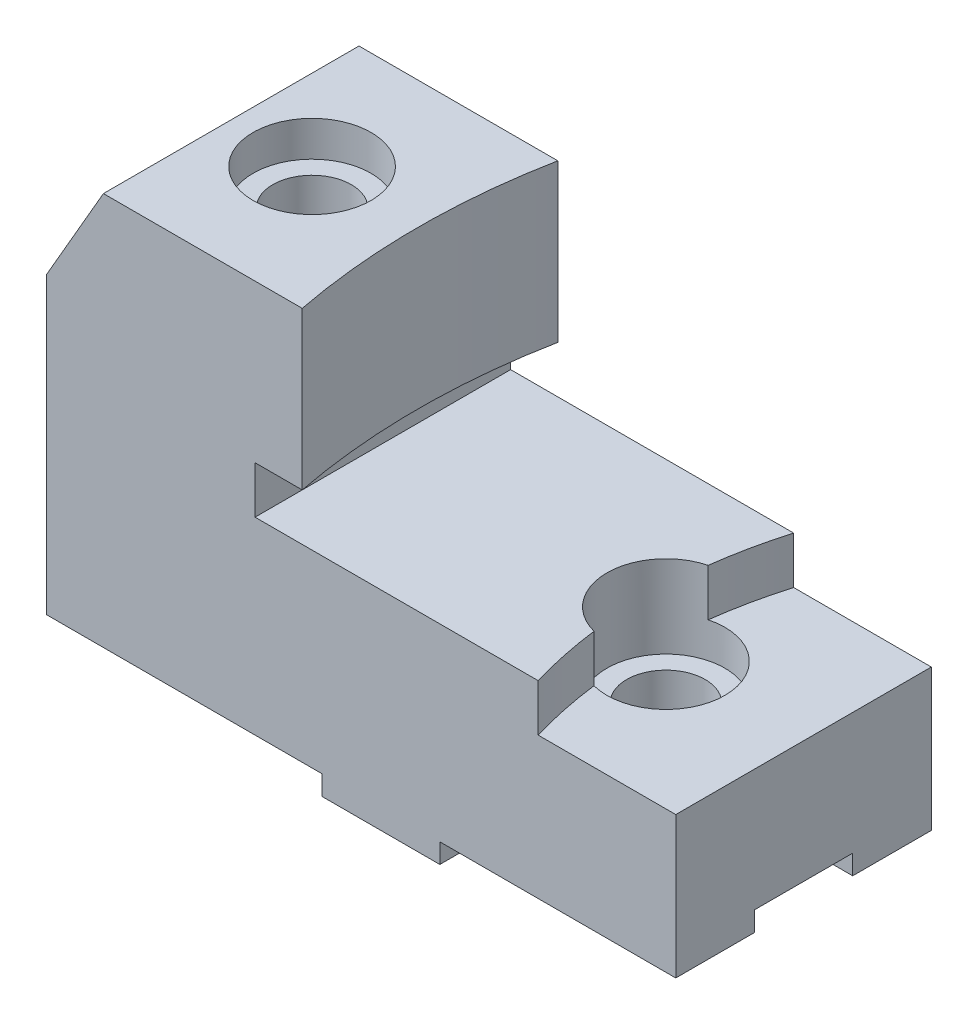
ISO-10303-21;
HEADER;
FILE_DESCRIPTION(('STEP AP214'),'2;1');
FILE_NAME('part.step','',(''),(''),'','','');
FILE_SCHEMA(('AUTOMOTIVE_DESIGN { 1 0 10303 214 1 1 1 1 }'));
ENDSEC;
DATA;
#1=APPLICATION_CONTEXT('core data for automotive mechanical design processes');
#2=APPLICATION_PROTOCOL_DEFINITION('international standard','automotive_design',2000,#1);
#3=PRODUCT_CONTEXT('',#1,'mechanical');
#4=PRODUCT('Part','Part','',(#3));
#5=PRODUCT_RELATED_PRODUCT_CATEGORY('part','',(#4));
#6=PRODUCT_DEFINITION_FORMATION('','',#4);
#7=PRODUCT_DEFINITION_CONTEXT('part definition',#1,'design');
#8=PRODUCT_DEFINITION('design','',#6,#7);
#9=PRODUCT_DEFINITION_SHAPE('','',#8);
#10=(LENGTH_UNIT() NAMED_UNIT(*) SI_UNIT(.MILLI.,.METRE.));
#11=(NAMED_UNIT(*) PLANE_ANGLE_UNIT() SI_UNIT($,.RADIAN.));
#12=(NAMED_UNIT(*) SI_UNIT($,.STERADIAN.) SOLID_ANGLE_UNIT());
#13=UNCERTAINTY_MEASURE_WITH_UNIT(LENGTH_MEASURE(1.E-05),#10,'distance_accuracy_value','');
#14=(GEOMETRIC_REPRESENTATION_CONTEXT(3) GLOBAL_UNCERTAINTY_ASSIGNED_CONTEXT((#13)) GLOBAL_UNIT_ASSIGNED_CONTEXT((#10,
#11,#12)) REPRESENTATION_CONTEXT('',''));
#15=CARTESIAN_POINT('',(0.,0.,0.));
#16=DIRECTION('',(0.,0.,1.));
#17=DIRECTION('',(1.,0.,0.));
#18=AXIS2_PLACEMENT_3D('',#15,#16,#17);
#19=CARTESIAN_POINT('',(235.312057364551,-289.269119345812,32.5));
#20=DIRECTION('',(0.,1.,0.));
#21=DIRECTION('',(-1.,0.,0.));
#22=AXIS2_PLACEMENT_3D('',#19,#20,#21);
#23=CYLINDRICAL_SURFACE('',#22,115.);
#24=CARTESIAN_POINT('',(235.312057364551,35.9999999999999,32.5));
#25=DIRECTION('',(0.,-1.,0.));
#26=DIRECTION('',(1.,0.,0.));
#27=AXIS2_PLACEMENT_3D('',#24,#25,#26);
#28=CIRCLE('',#27,115.);
#29=CARTESIAN_POINT('',(121.232279499362,36.,47.0191005998674));
#30=VERTEX_POINT('',#29);
#31=CARTESIAN_POINT('',(125.,36.,65.));
#32=VERTEX_POINT('',#31);
#33=EDGE_CURVE('E268',#30,#32,#28,.F.);
#34=ORIENTED_EDGE('',*,*,#33,.F.);
#35=DIRECTION('',(0.,1.,0.));
#36=VECTOR('',#35,1.);
#37=CARTESIAN_POINT('',(121.232279499362,42.,47.0191005998674));
#38=LINE('',#37,#36);
#39=CARTESIAN_POINT('',(121.232279499362,47.9999999999999,47.0191005998674));
#40=VERTEX_POINT('',#39);
#41=EDGE_CURVE('E479',#30,#40,#38,.T.);
#42=ORIENTED_EDGE('',*,*,#41,.T.);
#43=CARTESIAN_POINT('',(235.312057364551,47.9999999999998,32.5));
#44=DIRECTION('',(0.,1.,0.));
#45=DIRECTION('',(-1.,0.,0.));
#46=AXIS2_PLACEMENT_3D('',#43,#44,#45);
#47=CIRCLE('',#46,115.);
#48=CARTESIAN_POINT('',(125.,47.9999999999999,65.));
#49=VERTEX_POINT('',#48);
#50=EDGE_CURVE('E261',#40,#49,#47,.T.);
#51=ORIENTED_EDGE('',*,*,#50,.T.);
#52=DIRECTION('',(0.,1.,0.));
#53=VECTOR('',#52,1.);
#54=CARTESIAN_POINT('',(125.,48.,65.));
#55=LINE('',#54,#53);
#56=EDGE_CURVE('E332',#32,#49,#55,.T.);
#57=ORIENTED_EDGE('',*,*,#56,.F.);
#58=EDGE_LOOP('',(#34,#42,#51,#57));
#59=FACE_BOUND('',#58,.T.);
#60=ADVANCED_FACE('F39',(#59),#23,.F.);
#61=CARTESIAN_POINT('',(70.,0.,65.));
#62=DIRECTION('',(0.,1.,0.));
#63=DIRECTION('',(-1.,0.,0.));
#64=AXIS2_PLACEMENT_3D('',#61,#62,#63);
#65=PLANE('',#64);
#66=DIRECTION('',(0.,0.,-1.));
#67=VECTOR('',#66,1.);
#68=CARTESIAN_POINT('',(0.,0.,65.));
#69=LINE('',#68,#67);
#70=CARTESIAN_POINT('',(0.,0.,65.));
#71=VERTEX_POINT('',#70);
#72=CARTESIAN_POINT('',(0.,0.,45.));
#73=VERTEX_POINT('',#72);
#74=EDGE_CURVE('E217',#71,#73,#69,.T.);
#75=ORIENTED_EDGE('',*,*,#74,.T.);
#76=DIRECTION('',(1.,0.,0.));
#77=VECTOR('',#76,1.);
#78=CARTESIAN_POINT('',(70.,0.,45.));
#79=LINE('',#78,#77);
#80=CARTESIAN_POINT('',(70.,0.,45.));
#81=VERTEX_POINT('',#80);
#82=EDGE_CURVE('E179',#73,#81,#79,.T.);
#83=ORIENTED_EDGE('',*,*,#82,.T.);
#84=DIRECTION('',(0.,0.,-1.));
#85=VECTOR('',#84,1.);
#86=CARTESIAN_POINT('',(70.,0.,65.));
#87=LINE('',#86,#85);
#88=CARTESIAN_POINT('',(70.,0.,65.));
#89=VERTEX_POINT('',#88);
#90=EDGE_CURVE('E48',#89,#81,#87,.T.);
#91=ORIENTED_EDGE('',*,*,#90,.F.);
#92=DIRECTION('',(1.,0.,0.));
#93=VECTOR('',#92,1.);
#94=CARTESIAN_POINT('',(70.,0.,65.));
#95=LINE('',#94,#93);
#96=EDGE_CURVE('E213',#71,#89,#95,.T.);
#97=ORIENTED_EDGE('',*,*,#96,.F.);
#98=EDGE_LOOP('',(#75,#83,#91,#97));
#99=FACE_BOUND('',#98,.T.);
#100=ADVANCED_FACE('F368',(#99),#65,.F.);
#101=CARTESIAN_POINT('',(70.,0.,65.));
#102=DIRECTION('',(1.,0.,0.));
#103=DIRECTION('',(0.,0.,-1.));
#104=AXIS2_PLACEMENT_3D('',#101,#102,#103);
#105=PLANE('',#104);
#106=ORIENTED_EDGE('',*,*,#90,.T.);
#107=DIRECTION('',(0.,-1.,0.));
#108=VECTOR('',#107,1.);
#109=CARTESIAN_POINT('',(70.,0.,45.));
#110=LINE('',#109,#108);
#111=CARTESIAN_POINT('',(70.,-5.00000000000001,45.));
#112=VERTEX_POINT('',#111);
#113=EDGE_CURVE('E313',#81,#112,#110,.T.);
#114=ORIENTED_EDGE('',*,*,#113,.T.);
#115=DIRECTION('',(0.,0.,-1.));
#116=VECTOR('',#115,1.);
#117=CARTESIAN_POINT('',(70.,-5.00000000000001,65.));
#118=LINE('',#117,#116);
#119=CARTESIAN_POINT('',(70.,-5.00000000000001,65.));
#120=VERTEX_POINT('',#119);
#121=EDGE_CURVE('E241',#120,#112,#118,.T.);
#122=ORIENTED_EDGE('',*,*,#121,.F.);
#123=DIRECTION('',(0.,-1.,0.));
#124=VECTOR('',#123,1.);
#125=CARTESIAN_POINT('',(70.,0.,65.));
#126=LINE('',#125,#124);
#127=EDGE_CURVE('E124',#89,#120,#126,.T.);
#128=ORIENTED_EDGE('',*,*,#127,.F.);
#129=EDGE_LOOP('',(#106,#114,#122,#128));
#130=FACE_BOUND('',#129,.T.);
#131=ADVANCED_FACE('F371',(#130),#105,.F.);
#132=CARTESIAN_POINT('',(70.,-5.00000000000001,65.));
#133=DIRECTION('',(0.,1.,0.));
#134=DIRECTION('',(0.,0.,1.));
#135=AXIS2_PLACEMENT_3D('',#132,#133,#134);
#136=PLANE('',#135);
#137=ORIENTED_EDGE('',*,*,#121,.T.);
#138=DIRECTION('',(1.,0.,0.));
#139=VECTOR('',#138,1.);
#140=CARTESIAN_POINT('',(70.,-5.00000000000001,45.));
#141=LINE('',#140,#139);
#142=CARTESIAN_POINT('',(100.,-5.00000000000001,45.));
#143=VERTEX_POINT('',#142);
#144=EDGE_CURVE('E311',#112,#143,#141,.T.);
#145=ORIENTED_EDGE('',*,*,#144,.T.);
#146=DIRECTION('',(0.,0.,-1.));
#147=VECTOR('',#146,1.);
#148=CARTESIAN_POINT('',(100.,-5.00000000000001,65.));
#149=LINE('',#148,#147);
#150=CARTESIAN_POINT('',(100.,-5.00000000000001,65.));
#151=VERTEX_POINT('',#150);
#152=EDGE_CURVE('E240',#151,#143,#149,.T.);
#153=ORIENTED_EDGE('',*,*,#152,.F.);
#154=DIRECTION('',(1.,0.,0.));
#155=VECTOR('',#154,1.);
#156=CARTESIAN_POINT('',(70.,-5.00000000000001,65.));
#157=LINE('',#156,#155);
#158=EDGE_CURVE('E322',#120,#151,#157,.T.);
#159=ORIENTED_EDGE('',*,*,#158,.F.);
#160=EDGE_LOOP('',(#137,#145,#153,#159));
#161=FACE_BOUND('',#160,.T.);
#162=ADVANCED_FACE('F374',(#161),#136,.F.);
#163=CARTESIAN_POINT('',(100.,-5.00000000000001,65.));
#164=DIRECTION('',(-1.,0.,0.));
#165=DIRECTION('',(0.,0.,1.));
#166=AXIS2_PLACEMENT_3D('',#163,#164,#165);
#167=PLANE('',#166);
#168=ORIENTED_EDGE('',*,*,#152,.T.);
#169=DIRECTION('',(0.,1.,0.));
#170=VECTOR('',#169,1.);
#171=CARTESIAN_POINT('',(100.,-5.00000000000001,45.));
#172=LINE('',#171,#170);
#173=CARTESIAN_POINT('',(100.,0.,45.));
#174=VERTEX_POINT('',#173);
#175=EDGE_CURVE('E308',#143,#174,#172,.T.);
#176=ORIENTED_EDGE('',*,*,#175,.T.);
#177=DIRECTION('',(0.,0.,-1.));
#178=VECTOR('',#177,1.);
#179=CARTESIAN_POINT('',(100.,0.,65.));
#180=LINE('',#179,#178);
#181=CARTESIAN_POINT('',(100.,0.,65.));
#182=VERTEX_POINT('',#181);
#183=EDGE_CURVE('E231',#182,#174,#180,.T.);
#184=ORIENTED_EDGE('',*,*,#183,.F.);
#185=DIRECTION('',(0.,1.,0.));
#186=VECTOR('',#185,1.);
#187=CARTESIAN_POINT('',(100.,-5.00000000000001,65.));
#188=LINE('',#187,#186);
#189=EDGE_CURVE('E324',#151,#182,#188,.T.);
#190=ORIENTED_EDGE('',*,*,#189,.F.);
#191=EDGE_LOOP('',(#168,#176,#184,#190));
#192=FACE_BOUND('',#191,.T.);
#193=ADVANCED_FACE('F382',(#192),#167,.F.);
#194=CARTESIAN_POINT('',(160.,0.,65.));
#195=DIRECTION('',(0.,1.,0.));
#196=DIRECTION('',(-1.,0.,0.));
#197=AXIS2_PLACEMENT_3D('',#194,#195,#196);
#198=PLANE('',#197);
#199=ORIENTED_EDGE('',*,*,#183,.T.);
#200=DIRECTION('',(1.,0.,0.));
#201=VECTOR('',#200,1.);
#202=CARTESIAN_POINT('',(160.,0.,45.));
#203=LINE('',#202,#201);
#204=CARTESIAN_POINT('',(160.,0.,45.));
#205=VERTEX_POINT('',#204);
#206=EDGE_CURVE('E304',#174,#205,#203,.T.);
#207=ORIENTED_EDGE('',*,*,#206,.T.);
#208=DIRECTION('',(0.,0.,-1.));
#209=VECTOR('',#208,1.);
#210=CARTESIAN_POINT('',(160.,0.,65.));
#211=LINE('',#210,#209);
#212=CARTESIAN_POINT('',(160.,0.,65.));
#213=VERTEX_POINT('',#212);
#214=EDGE_CURVE('E230',#213,#205,#211,.T.);
#215=ORIENTED_EDGE('',*,*,#214,.F.);
#216=DIRECTION('',(1.,0.,0.));
#217=VECTOR('',#216,1.);
#218=CARTESIAN_POINT('',(160.,0.,65.));
#219=LINE('',#218,#217);
#220=EDGE_CURVE('E323',#182,#213,#219,.T.);
#221=ORIENTED_EDGE('',*,*,#220,.F.);
#222=EDGE_LOOP('',(#199,#207,#215,#221));
#223=FACE_BOUND('',#222,.T.);
#224=ADVANCED_FACE('F390',(#223),#198,.F.);
#225=CARTESIAN_POINT('',(70.,0.,20.));
#226=VERTEX_POINT('',#225);
#227=CARTESIAN_POINT('',(70.,0.,0.));
#228=VERTEX_POINT('',#227);
#229=EDGE_CURVE('E242',#226,#228,#87,.T.);
#230=ORIENTED_EDGE('',*,*,#229,.F.);
#231=DIRECTION('',(-1.,0.,0.));
#232=VECTOR('',#231,1.);
#233=CARTESIAN_POINT('',(70.,0.,20.));
#234=LINE('',#233,#232);
#235=CARTESIAN_POINT('',(0.,0.,20.));
#236=VERTEX_POINT('',#235);
#237=EDGE_CURVE('E303',#226,#236,#234,.T.);
#238=ORIENTED_EDGE('',*,*,#237,.T.);
#239=CARTESIAN_POINT('',(0.,0.,0.));
#240=VERTEX_POINT('',#239);
#241=EDGE_CURVE('E112',#236,#240,#69,.T.);
#242=ORIENTED_EDGE('',*,*,#241,.T.);
#243=DIRECTION('',(1.,0.,0.));
#244=VECTOR('',#243,1.);
#245=CARTESIAN_POINT('',(70.,0.,0.));
#246=LINE('',#245,#244);
#247=EDGE_CURVE('E180',#240,#228,#246,.T.);
#248=ORIENTED_EDGE('',*,*,#247,.T.);
#249=EDGE_LOOP('',(#230,#238,#242,#248));
#250=FACE_BOUND('',#249,.T.);
#251=ADVANCED_FACE('F41',(#250),#65,.F.);
#252=CARTESIAN_POINT('',(70.,-5.00000000000001,20.));
#253=VERTEX_POINT('',#252);
#254=CARTESIAN_POINT('',(70.,-5.00000000000001,0.));
#255=VERTEX_POINT('',#254);
#256=EDGE_CURVE('E239',#253,#255,#118,.T.);
#257=ORIENTED_EDGE('',*,*,#256,.F.);
#258=DIRECTION('',(0.,1.,0.));
#259=VECTOR('',#258,1.);
#260=CARTESIAN_POINT('',(70.,0.,20.));
#261=LINE('',#260,#259);
#262=EDGE_CURVE('E297',#253,#226,#261,.T.);
#263=ORIENTED_EDGE('',*,*,#262,.T.);
#264=ORIENTED_EDGE('',*,*,#229,.T.);
#265=DIRECTION('',(0.,-1.,0.));
#266=VECTOR('',#265,1.);
#267=CARTESIAN_POINT('',(70.,0.,0.));
#268=LINE('',#267,#266);
#269=EDGE_CURVE('E177',#228,#255,#268,.T.);
#270=ORIENTED_EDGE('',*,*,#269,.T.);
#271=EDGE_LOOP('',(#257,#263,#264,#270));
#272=FACE_BOUND('',#271,.T.);
#273=ADVANCED_FACE('F446',(#272),#105,.F.);
#274=CARTESIAN_POINT('',(100.,-5.00000000000001,20.));
#275=VERTEX_POINT('',#274);
#276=CARTESIAN_POINT('',(100.,-5.00000000000001,0.));
#277=VERTEX_POINT('',#276);
#278=EDGE_CURVE('E236',#275,#277,#149,.T.);
#279=ORIENTED_EDGE('',*,*,#278,.F.);
#280=DIRECTION('',(-1.,0.,0.));
#281=VECTOR('',#280,1.);
#282=CARTESIAN_POINT('',(70.,-5.00000000000001,20.));
#283=LINE('',#282,#281);
#284=EDGE_CURVE('E300',#275,#253,#283,.T.);
#285=ORIENTED_EDGE('',*,*,#284,.T.);
#286=ORIENTED_EDGE('',*,*,#256,.T.);
#287=DIRECTION('',(1.,0.,0.));
#288=VECTOR('',#287,1.);
#289=CARTESIAN_POINT('',(70.,-5.00000000000001,0.));
#290=LINE('',#289,#288);
#291=EDGE_CURVE('E182',#255,#277,#290,.T.);
#292=ORIENTED_EDGE('',*,*,#291,.T.);
#293=EDGE_LOOP('',(#279,#285,#286,#292));
#294=FACE_BOUND('',#293,.T.);
#295=ADVANCED_FACE('F453',(#294),#136,.F.);
#296=CARTESIAN_POINT('',(100.,0.,20.));
#297=VERTEX_POINT('',#296);
#298=CARTESIAN_POINT('',(100.,0.,0.));
#299=VERTEX_POINT('',#298);
#300=EDGE_CURVE('E235',#297,#299,#180,.T.);
#301=ORIENTED_EDGE('',*,*,#300,.F.);
#302=DIRECTION('',(0.,-1.,0.));
#303=VECTOR('',#302,1.);
#304=CARTESIAN_POINT('',(100.,-5.00000000000001,20.));
#305=LINE('',#304,#303);
#306=EDGE_CURVE('E295',#297,#275,#305,.T.);
#307=ORIENTED_EDGE('',*,*,#306,.T.);
#308=ORIENTED_EDGE('',*,*,#278,.T.);
#309=DIRECTION('',(0.,1.,0.));
#310=VECTOR('',#309,1.);
#311=CARTESIAN_POINT('',(100.,-5.00000000000001,0.));
#312=LINE('',#311,#310);
#313=EDGE_CURVE('E187',#277,#299,#312,.T.);
#314=ORIENTED_EDGE('',*,*,#313,.T.);
#315=EDGE_LOOP('',(#301,#307,#308,#314));
#316=FACE_BOUND('',#315,.T.);
#317=ADVANCED_FACE('F458',(#316),#167,.F.);
#318=CARTESIAN_POINT('',(160.,0.,20.));
#319=VERTEX_POINT('',#318);
#320=CARTESIAN_POINT('',(160.,0.,0.));
#321=VERTEX_POINT('',#320);
#322=EDGE_CURVE('E226',#319,#321,#211,.T.);
#323=ORIENTED_EDGE('',*,*,#322,.F.);
#324=DIRECTION('',(-1.,0.,0.));
#325=VECTOR('',#324,1.);
#326=CARTESIAN_POINT('',(160.,0.,20.));
#327=LINE('',#326,#325);
#328=EDGE_CURVE('E290',#319,#297,#327,.T.);
#329=ORIENTED_EDGE('',*,*,#328,.T.);
#330=ORIENTED_EDGE('',*,*,#300,.T.);
#331=DIRECTION('',(1.,0.,0.));
#332=VECTOR('',#331,1.);
#333=CARTESIAN_POINT('',(160.,0.,0.));
#334=LINE('',#333,#332);
#335=EDGE_CURVE('E186',#299,#321,#334,.T.);
#336=ORIENTED_EDGE('',*,*,#335,.T.);
#337=EDGE_LOOP('',(#323,#329,#330,#336));
#338=FACE_BOUND('',#337,.T.);
#339=ADVANCED_FACE('F461',(#338),#198,.F.);
#340=CARTESIAN_POINT('',(160.,36.,65.));
#341=DIRECTION('',(-1.,0.,0.));
#342=DIRECTION('',(0.,0.,1.));
#343=AXIS2_PLACEMENT_3D('',#340,#341,#342);
#344=PLANE('',#343);
#345=ORIENTED_EDGE('',*,*,#214,.T.);
#346=DIRECTION('',(0.,-1.,0.));
#347=VECTOR('',#346,1.);
#348=CARTESIAN_POINT('',(160.,0.,45.));
#349=LINE('',#348,#347);
#350=CARTESIAN_POINT('',(160.,4.99999999999999,45.));
#351=VERTEX_POINT('',#350);
#352=EDGE_CURVE('E280',#351,#205,#349,.T.);
#353=ORIENTED_EDGE('',*,*,#352,.F.);
#354=DIRECTION('',(0.,0.,1.));
#355=VECTOR('',#354,1.);
#356=CARTESIAN_POINT('',(160.,4.99999999999999,45.));
#357=LINE('',#356,#355);
#358=CARTESIAN_POINT('',(160.,4.99999999999999,20.));
#359=VERTEX_POINT('',#358);
#360=EDGE_CURVE('E285',#359,#351,#357,.T.);
#361=ORIENTED_EDGE('',*,*,#360,.F.);
#362=DIRECTION('',(0.,1.,0.));
#363=VECTOR('',#362,1.);
#364=CARTESIAN_POINT('',(160.,0.,20.));
#365=LINE('',#364,#363);
#366=EDGE_CURVE('E271',#319,#359,#365,.T.);
#367=ORIENTED_EDGE('',*,*,#366,.F.);
#368=ORIENTED_EDGE('',*,*,#322,.T.);
#369=DIRECTION('',(0.,1.,0.));
#370=VECTOR('',#369,1.);
#371=CARTESIAN_POINT('',(160.,36.,0.));
#372=LINE('',#371,#370);
#373=CARTESIAN_POINT('',(160.,36.,0.));
#374=VERTEX_POINT('',#373);
#375=EDGE_CURVE('E195',#321,#374,#372,.T.);
#376=ORIENTED_EDGE('',*,*,#375,.T.);
#377=DIRECTION('',(0.,0.,-1.));
#378=VECTOR('',#377,1.);
#379=CARTESIAN_POINT('',(160.,36.,65.));
#380=LINE('',#379,#378);
#381=CARTESIAN_POINT('',(160.,36.,65.));
#382=VERTEX_POINT('',#381);
#383=EDGE_CURVE('E225',#382,#374,#380,.T.);
#384=ORIENTED_EDGE('',*,*,#383,.F.);
#385=DIRECTION('',(0.,1.,0.));
#386=VECTOR('',#385,1.);
#387=CARTESIAN_POINT('',(160.,36.,65.));
#388=LINE('',#387,#386);
#389=EDGE_CURVE('E330',#213,#382,#388,.T.);
#390=ORIENTED_EDGE('',*,*,#389,.F.);
#391=EDGE_LOOP('',(#345,#353,#361,#367,#368,#376,#384,#390));
#392=FACE_BOUND('',#391,.T.);
#393=ADVANCED_FACE('F395',(#392),#344,.F.);
#394=CARTESIAN_POINT('',(125.,36.,65.));
#395=DIRECTION('',(0.,-1.,0.));
#396=DIRECTION('',(1.,0.,0.));
#397=AXIS2_PLACEMENT_3D('',#394,#395,#396);
#398=PLANE('',#397);
#399=CARTESIAN_POINT('',(125.,36.,0.));
#400=VERTEX_POINT('',#399);
#401=CARTESIAN_POINT('',(121.232279499362,36.,17.9808994001326));
#402=VERTEX_POINT('',#401);
#403=EDGE_CURVE('E270',#400,#402,#28,.F.);
#404=ORIENTED_EDGE('',*,*,#403,.T.);
#405=CARTESIAN_POINT('',(125.,36.,32.5));
#406=DIRECTION('',(0.,1.,0.));
#407=DIRECTION('',(0.,0.,1.));
#408=AXIS2_PLACEMENT_3D('',#405,#406,#407);
#409=CIRCLE('',#408,15.);
#410=EDGE_CURVE('E258',#30,#402,#409,.T.);
#411=ORIENTED_EDGE('',*,*,#410,.F.);
#412=ORIENTED_EDGE('',*,*,#33,.T.);
#413=DIRECTION('',(-1.,0.,0.));
#414=VECTOR('',#413,1.);
#415=CARTESIAN_POINT('',(125.,36.,65.));
#416=LINE('',#415,#414);
#417=EDGE_CURVE('E329',#382,#32,#416,.T.);
#418=ORIENTED_EDGE('',*,*,#417,.F.);
#419=ORIENTED_EDGE('',*,*,#383,.T.);
#420=DIRECTION('',(-1.,0.,0.));
#421=VECTOR('',#420,1.);
#422=CARTESIAN_POINT('',(125.,36.,0.));
#423=LINE('',#422,#421);
#424=EDGE_CURVE('E191',#374,#400,#423,.T.);
#425=ORIENTED_EDGE('',*,*,#424,.T.);
#426=EDGE_LOOP('',(#404,#411,#412,#418,#419,#425));
#427=FACE_BOUND('',#426,.T.);
#428=ADVANCED_FACE('F399',(#427),#398,.F.);
#429=CARTESIAN_POINT('',(65.,48.,65.));
#430=DIRECTION('',(0.,-1.,0.));
#431=DIRECTION('',(1.,0.,0.));
#432=AXIS2_PLACEMENT_3D('',#429,#430,#431);
#433=PLANE('',#432);
#434=ORIENTED_EDGE('',*,*,#50,.F.);
#435=CARTESIAN_POINT('',(125.,47.9999999999999,32.5));
#436=DIRECTION('',(0.,1.,0.));
#437=DIRECTION('',(-1.,0.,0.));
#438=AXIS2_PLACEMENT_3D('',#435,#436,#437);
#439=CIRCLE('',#438,15.);
#440=CARTESIAN_POINT('',(121.232279499362,47.9999999999999,17.9808994001326));
#441=VERTEX_POINT('',#440);
#442=EDGE_CURVE('E476',#441,#40,#439,.T.);
#443=ORIENTED_EDGE('',*,*,#442,.F.);
#444=CARTESIAN_POINT('',(125.,47.9999999999999,0.));
#445=VERTEX_POINT('',#444);
#446=EDGE_CURVE('E266',#445,#441,#47,.T.);
#447=ORIENTED_EDGE('',*,*,#446,.F.);
#448=DIRECTION('',(-1.,0.,0.));
#449=VECTOR('',#448,1.);
#450=CARTESIAN_POINT('',(65.,48.,0.));
#451=LINE('',#450,#449);
#452=CARTESIAN_POINT('',(53.,48.,0.));
#453=VERTEX_POINT('',#452);
#454=EDGE_CURVE('E196',#445,#453,#451,.T.);
#455=ORIENTED_EDGE('',*,*,#454,.T.);
#456=DIRECTION('',(0.,0.,-1.));
#457=VECTOR('',#456,1.);
#458=CARTESIAN_POINT('',(53.,48.,65.));
#459=LINE('',#458,#457);
#460=CARTESIAN_POINT('',(53.,48.,65.));
#461=VERTEX_POINT('',#460);
#462=EDGE_CURVE('E222',#461,#453,#459,.T.);
#463=ORIENTED_EDGE('',*,*,#462,.F.);
#464=DIRECTION('',(-1.,0.,0.));
#465=VECTOR('',#464,1.);
#466=CARTESIAN_POINT('',(65.,48.,65.));
#467=LINE('',#466,#465);
#468=EDGE_CURVE('E335',#49,#461,#467,.T.);
#469=ORIENTED_EDGE('',*,*,#468,.F.);
#470=EDGE_LOOP('',(#434,#443,#447,#455,#463,#469));
#471=FACE_BOUND('',#470,.T.);
#472=ADVANCED_FACE('F505',(#471),#433,.F.);
#473=CARTESIAN_POINT('',(53.,48.,65.));
#474=DIRECTION('',(-1.,0.,0.));
#475=DIRECTION('',(0.,0.,1.));
#476=AXIS2_PLACEMENT_3D('',#473,#474,#475);
#477=PLANE('',#476);
#478=DIRECTION('',(0.,1.,0.));
#479=VECTOR('',#478,1.);
#480=CARTESIAN_POINT('',(53.,48.,0.));
#481=LINE('',#480,#479);
#482=CARTESIAN_POINT('',(53.,60.,0.));
#483=VERTEX_POINT('',#482);
#484=EDGE_CURVE('E202',#453,#483,#481,.T.);
#485=ORIENTED_EDGE('',*,*,#484,.T.);
#486=DIRECTION('',(0.,0.,-1.));
#487=VECTOR('',#486,1.);
#488=CARTESIAN_POINT('',(53.,60.,65.));
#489=LINE('',#488,#487);
#490=CARTESIAN_POINT('',(53.,60.,65.));
#491=VERTEX_POINT('',#490);
#492=EDGE_CURVE('E166',#491,#483,#489,.T.);
#493=ORIENTED_EDGE('',*,*,#492,.F.);
#494=DIRECTION('',(0.,1.,0.));
#495=VECTOR('',#494,1.);
#496=CARTESIAN_POINT('',(53.,48.,65.));
#497=LINE('',#496,#495);
#498=EDGE_CURVE('E340',#461,#491,#497,.T.);
#499=ORIENTED_EDGE('',*,*,#498,.F.);
#500=ORIENTED_EDGE('',*,*,#462,.T.);
#501=EDGE_LOOP('',(#485,#493,#499,#500));
#502=FACE_BOUND('',#501,.T.);
#503=ADVANCED_FACE('F507',(#502),#477,.F.);
#504=CARTESIAN_POINT('',(53.,60.,65.));
#505=DIRECTION('',(0.,1.,0.));
#506=DIRECTION('',(0.,0.,1.));
#507=AXIS2_PLACEMENT_3D('',#504,#505,#506);
#508=PLANE('',#507);
#509=DIRECTION('',(1.,0.,0.));
#510=VECTOR('',#509,1.);
#511=CARTESIAN_POINT('',(53.,60.,0.));
#512=LINE('',#511,#510);
#513=CARTESIAN_POINT('',(65.,60.,0.));
#514=VERTEX_POINT('',#513);
#515=EDGE_CURVE('E203',#483,#514,#512,.T.);
#516=ORIENTED_EDGE('',*,*,#515,.T.);
#517=CARTESIAN_POINT('',(231.864465959652,60.,32.5));
#518=DIRECTION('',(0.,1.,0.));
#519=DIRECTION('',(0.,0.,1.));
#520=AXIS2_PLACEMENT_3D('',#517,#518,#519);
#521=CIRCLE('',#520,170.);
#522=CARTESIAN_POINT('',(65.,60.,65.));
#523=VERTEX_POINT('',#522);
#524=EDGE_CURVE('E255',#523,#514,#521,.F.);
#525=ORIENTED_EDGE('',*,*,#524,.F.);
#526=DIRECTION('',(1.,0.,0.));
#527=VECTOR('',#526,1.);
#528=CARTESIAN_POINT('',(53.,60.,65.));
#529=LINE('',#528,#527);
#530=EDGE_CURVE('E339',#491,#523,#529,.T.);
#531=ORIENTED_EDGE('',*,*,#530,.F.);
#532=ORIENTED_EDGE('',*,*,#492,.T.);
#533=EDGE_LOOP('',(#516,#525,#531,#532));
#534=FACE_BOUND('',#533,.T.);
#535=ADVANCED_FACE('F348',(#534),#508,.F.);
#536=CARTESIAN_POINT('',(14.4337567297407,100.,65.));
#537=DIRECTION('',(0.,-1.,0.));
#538=DIRECTION('',(1.,0.,0.));
#539=AXIS2_PLACEMENT_3D('',#536,#537,#538);
#540=PLANE('',#539);
#541=CARTESIAN_POINT('',(35.,100.,32.5));
#542=DIRECTION('',(0.,1.,0.));
#543=DIRECTION('',(0.,0.,1.));
#544=AXIS2_PLACEMENT_3D('',#541,#542,#543);
#545=CIRCLE('',#544,15.);
#546=CARTESIAN_POINT('',(35.,100.,47.5));
#547=VERTEX_POINT('',#546);
#548=EDGE_CURVE('E491',#547,#547,#545,.T.);
#549=ORIENTED_EDGE('',*,*,#548,.F.);
#550=EDGE_LOOP('',(#549));
#551=FACE_BOUND('',#550,.T.);
#552=DIRECTION('',(-1.,0.,0.));
#553=VECTOR('',#552,1.);
#554=CARTESIAN_POINT('',(14.4337567297407,100.,65.));
#555=LINE('',#554,#553);
#556=CARTESIAN_POINT('',(65.,100.,65.));
#557=VERTEX_POINT('',#556);
#558=CARTESIAN_POINT('',(14.4337567297407,100.,65.));
#559=VERTEX_POINT('',#558);
#560=EDGE_CURVE('E149',#557,#559,#555,.T.);
#561=ORIENTED_EDGE('',*,*,#560,.F.);
#562=CARTESIAN_POINT('',(231.864465959652,99.9999999999999,32.5));
#563=DIRECTION('',(0.,1.,0.));
#564=DIRECTION('',(-1.,0.,0.));
#565=AXIS2_PLACEMENT_3D('',#562,#563,#564);
#566=CIRCLE('',#565,170.);
#567=CARTESIAN_POINT('',(65.,100.,0.));
#568=VERTEX_POINT('',#567);
#569=EDGE_CURVE('E250',#568,#557,#566,.T.);
#570=ORIENTED_EDGE('',*,*,#569,.F.);
#571=DIRECTION('',(-1.,0.,0.));
#572=VECTOR('',#571,1.);
#573=CARTESIAN_POINT('',(14.4337567297407,100.,0.));
#574=LINE('',#573,#572);
#575=CARTESIAN_POINT('',(14.4337567297407,100.,0.));
#576=VERTEX_POINT('',#575);
#577=EDGE_CURVE('E164',#568,#576,#574,.T.);
#578=ORIENTED_EDGE('',*,*,#577,.T.);
#579=DIRECTION('',(0.,0.,-1.));
#580=VECTOR('',#579,1.);
#581=CARTESIAN_POINT('',(14.4337567297407,100.,65.));
#582=LINE('',#581,#580);
#583=EDGE_CURVE('E162',#559,#576,#582,.T.);
#584=ORIENTED_EDGE('',*,*,#583,.F.);
#585=EDGE_LOOP('',(#561,#570,#578,#584));
#586=FACE_BOUND('',#585,.T.);
#587=ADVANCED_FACE('F161',(#551,#586),#540,.F.);
#588=CARTESIAN_POINT('',(0.,75.,65.));
#589=DIRECTION('',(0.866025403784438,-0.500000000000001,0.));
#590=DIRECTION('',(0.500000000000001,0.866025403784438,0.));
#591=AXIS2_PLACEMENT_3D('',#588,#589,#590);
#592=PLANE('',#591);
#593=DIRECTION('',(-0.500000000000001,-0.866025403784438,0.));
#594=VECTOR('',#593,1.);
#595=CARTESIAN_POINT('',(0.,75.,0.));
#596=LINE('',#595,#594);
#597=CARTESIAN_POINT('',(0.,75.,0.));
#598=VERTEX_POINT('',#597);
#599=EDGE_CURVE('E212',#576,#598,#596,.T.);
#600=ORIENTED_EDGE('',*,*,#599,.T.);
#601=DIRECTION('',(0.,0.,-1.));
#602=VECTOR('',#601,1.);
#603=CARTESIAN_POINT('',(0.,75.,65.));
#604=LINE('',#603,#602);
#605=CARTESIAN_POINT('',(0.,75.,65.));
#606=VERTEX_POINT('',#605);
#607=EDGE_CURVE('E169',#606,#598,#604,.T.);
#608=ORIENTED_EDGE('',*,*,#607,.F.);
#609=DIRECTION('',(-0.500000000000001,-0.866025403784438,0.));
#610=VECTOR('',#609,1.);
#611=CARTESIAN_POINT('',(0.,75.,65.));
#612=LINE('',#611,#610);
#613=EDGE_CURVE('E155',#559,#606,#612,.T.);
#614=ORIENTED_EDGE('',*,*,#613,.F.);
#615=ORIENTED_EDGE('',*,*,#583,.T.);
#616=EDGE_LOOP('',(#600,#608,#614,#615));
#617=FACE_BOUND('',#616,.T.);
#618=ADVANCED_FACE('F171',(#617),#592,.F.);
#619=CARTESIAN_POINT('',(0.,0.,65.));
#620=DIRECTION('',(1.,0.,0.));
#621=DIRECTION('',(0.,0.,-1.));
#622=AXIS2_PLACEMENT_3D('',#619,#620,#621);
#623=PLANE('',#622);
#624=DIRECTION('',(0.,0.,1.));
#625=VECTOR('',#624,1.);
#626=CARTESIAN_POINT('',(0.,4.99999999999999,45.));
#627=LINE('',#626,#625);
#628=CARTESIAN_POINT('',(0.,4.99999999999999,20.));
#629=VERTEX_POINT('',#628);
#630=CARTESIAN_POINT('',(0.,4.99999999999999,45.));
#631=VERTEX_POINT('',#630);
#632=EDGE_CURVE('E57',#629,#631,#627,.T.);
#633=ORIENTED_EDGE('',*,*,#632,.T.);
#634=DIRECTION('',(0.,-1.,0.));
#635=VECTOR('',#634,1.);
#636=CARTESIAN_POINT('',(0.,0.,45.));
#637=LINE('',#636,#635);
#638=EDGE_CURVE('E274',#631,#73,#637,.T.);
#639=ORIENTED_EDGE('',*,*,#638,.T.);
#640=ORIENTED_EDGE('',*,*,#74,.F.);
#641=DIRECTION('',(0.,-1.,0.));
#642=VECTOR('',#641,1.);
#643=CARTESIAN_POINT('',(0.,0.,65.));
#644=LINE('',#643,#642);
#645=EDGE_CURVE('E63',#606,#71,#644,.T.);
#646=ORIENTED_EDGE('',*,*,#645,.F.);
#647=ORIENTED_EDGE('',*,*,#607,.T.);
#648=DIRECTION('',(0.,-1.,0.));
#649=VECTOR('',#648,1.);
#650=CARTESIAN_POINT('',(0.,0.,0.));
#651=LINE('',#650,#649);
#652=EDGE_CURVE('E214',#598,#240,#651,.T.);
#653=ORIENTED_EDGE('',*,*,#652,.T.);
#654=ORIENTED_EDGE('',*,*,#241,.F.);
#655=DIRECTION('',(0.,1.,0.));
#656=VECTOR('',#655,1.);
#657=CARTESIAN_POINT('',(0.,0.,20.));
#658=LINE('',#657,#656);
#659=EDGE_CURVE('E11',#236,#629,#658,.T.);
#660=ORIENTED_EDGE('',*,*,#659,.T.);
#661=EDGE_LOOP('',(#633,#639,#640,#646,#647,#653,#654,#660));
#662=FACE_BOUND('',#661,.T.);
#663=ADVANCED_FACE('F365',(#662),#623,.F.);
#664=CARTESIAN_POINT('',(0.,0.,65.));
#665=DIRECTION('',(0.,0.,-1.));
#666=DIRECTION('',(-1.,0.,0.));
#667=AXIS2_PLACEMENT_3D('',#664,#665,#666);
#668=PLANE('',#667);
#669=ORIENTED_EDGE('',*,*,#96,.T.);
#670=ORIENTED_EDGE('',*,*,#127,.T.);
#671=ORIENTED_EDGE('',*,*,#158,.T.);
#672=ORIENTED_EDGE('',*,*,#189,.T.);
#673=ORIENTED_EDGE('',*,*,#220,.T.);
#674=ORIENTED_EDGE('',*,*,#389,.T.);
#675=ORIENTED_EDGE('',*,*,#417,.T.);
#676=ORIENTED_EDGE('',*,*,#56,.T.);
#677=ORIENTED_EDGE('',*,*,#468,.T.);
#678=ORIENTED_EDGE('',*,*,#498,.T.);
#679=ORIENTED_EDGE('',*,*,#530,.T.);
#680=DIRECTION('',(0.,1.,0.));
#681=VECTOR('',#680,1.);
#682=CARTESIAN_POINT('',(65.,100.,65.));
#683=LINE('',#682,#681);
#684=EDGE_CURVE('E157',#523,#557,#683,.T.);
#685=ORIENTED_EDGE('',*,*,#684,.T.);
#686=ORIENTED_EDGE('',*,*,#560,.T.);
#687=ORIENTED_EDGE('',*,*,#613,.T.);
#688=ORIENTED_EDGE('',*,*,#645,.T.);
#689=EDGE_LOOP('',(#669,#670,#671,#672,#673,#674,#675,#676,#677,#678,#679,#685,#686,#687,#688));
#690=FACE_BOUND('',#689,.T.);
#691=ADVANCED_FACE('F148',(#690),#668,.F.);
#692=CARTESIAN_POINT('',(0.,0.,0.));
#693=DIRECTION('',(0.,0.,-1.));
#694=DIRECTION('',(-1.,0.,0.));
#695=AXIS2_PLACEMENT_3D('',#692,#693,#694);
#696=PLANE('',#695);
#697=ORIENTED_EDGE('',*,*,#247,.F.);
#698=ORIENTED_EDGE('',*,*,#652,.F.);
#699=ORIENTED_EDGE('',*,*,#599,.F.);
#700=ORIENTED_EDGE('',*,*,#577,.F.);
#701=DIRECTION('',(0.,1.,0.));
#702=VECTOR('',#701,1.);
#703=CARTESIAN_POINT('',(65.,100.,0.));
#704=LINE('',#703,#702);
#705=EDGE_CURVE('E210',#514,#568,#704,.T.);
#706=ORIENTED_EDGE('',*,*,#705,.F.);
#707=ORIENTED_EDGE('',*,*,#515,.F.);
#708=ORIENTED_EDGE('',*,*,#484,.F.);
#709=ORIENTED_EDGE('',*,*,#454,.F.);
#710=DIRECTION('',(0.,1.,0.));
#711=VECTOR('',#710,1.);
#712=CARTESIAN_POINT('',(125.,48.,0.));
#713=LINE('',#712,#711);
#714=EDGE_CURVE('E200',#400,#445,#713,.T.);
#715=ORIENTED_EDGE('',*,*,#714,.F.);
#716=ORIENTED_EDGE('',*,*,#424,.F.);
#717=ORIENTED_EDGE('',*,*,#375,.F.);
#718=ORIENTED_EDGE('',*,*,#335,.F.);
#719=ORIENTED_EDGE('',*,*,#313,.F.);
#720=ORIENTED_EDGE('',*,*,#291,.F.);
#721=ORIENTED_EDGE('',*,*,#269,.F.);
#722=EDGE_LOOP('',(#697,#698,#699,#700,#706,#707,#708,#709,#715,#716,#717,#718,#719,#720,#721));
#723=FACE_BOUND('',#722,.T.);
#724=ADVANCED_FACE('F360',(#723),#696,.T.);
#725=CARTESIAN_POINT('',(0.,0.,45.));
#726=DIRECTION('',(0.,0.,1.));
#727=DIRECTION('',(1.,0.,0.));
#728=AXIS2_PLACEMENT_3D('',#725,#726,#727);
#729=PLANE('',#728);
#730=ORIENTED_EDGE('',*,*,#638,.F.);
#731=DIRECTION('',(1.,0.,0.));
#732=VECTOR('',#731,1.);
#733=CARTESIAN_POINT('',(0.,4.99999999999999,45.));
#734=LINE('',#733,#732);
#735=EDGE_CURVE('E287',#631,#351,#734,.T.);
#736=ORIENTED_EDGE('',*,*,#735,.T.);
#737=ORIENTED_EDGE('',*,*,#352,.T.);
#738=ORIENTED_EDGE('',*,*,#206,.F.);
#739=ORIENTED_EDGE('',*,*,#175,.F.);
#740=ORIENTED_EDGE('',*,*,#144,.F.);
#741=ORIENTED_EDGE('',*,*,#113,.F.);
#742=ORIENTED_EDGE('',*,*,#82,.F.);
#743=EDGE_LOOP('',(#730,#736,#737,#738,#739,#740,#741,#742));
#744=FACE_BOUND('',#743,.T.);
#745=ADVANCED_FACE('F439',(#744),#729,.F.);
#746=CARTESIAN_POINT('',(0.,0.,20.));
#747=DIRECTION('',(0.,0.,-1.));
#748=DIRECTION('',(-1.,0.,0.));
#749=AXIS2_PLACEMENT_3D('',#746,#747,#748);
#750=PLANE('',#749);
#751=ORIENTED_EDGE('',*,*,#262,.F.);
#752=ORIENTED_EDGE('',*,*,#284,.F.);
#753=ORIENTED_EDGE('',*,*,#306,.F.);
#754=ORIENTED_EDGE('',*,*,#328,.F.);
#755=ORIENTED_EDGE('',*,*,#366,.T.);
#756=DIRECTION('',(1.,0.,0.));
#757=VECTOR('',#756,1.);
#758=CARTESIAN_POINT('',(0.,4.99999999999999,20.));
#759=LINE('',#758,#757);
#760=EDGE_CURVE('E276',#629,#359,#759,.T.);
#761=ORIENTED_EDGE('',*,*,#760,.F.);
#762=ORIENTED_EDGE('',*,*,#659,.F.);
#763=ORIENTED_EDGE('',*,*,#237,.F.);
#764=EDGE_LOOP('',(#751,#752,#753,#754,#755,#761,#762,#763));
#765=FACE_BOUND('',#764,.T.);
#766=ADVANCED_FACE('F443',(#765),#750,.F.);
#767=CARTESIAN_POINT('',(0.,4.99999999999999,45.));
#768=DIRECTION('',(0.,1.,0.));
#769=DIRECTION('',(0.,0.,1.));
#770=AXIS2_PLACEMENT_3D('',#767,#768,#769);
#771=PLANE('',#770);
#772=CARTESIAN_POINT('',(35.,4.99999999999999,32.5));
#773=DIRECTION('',(0.,1.,0.));
#774=DIRECTION('',(0.,0.,1.));
#775=AXIS2_PLACEMENT_3D('',#772,#773,#774);
#776=CIRCLE('',#775,10.);
#777=CARTESIAN_POINT('',(35.,4.99999999999999,42.5));
#778=VERTEX_POINT('',#777);
#779=EDGE_CURVE('E43',#778,#778,#776,.T.);
#780=ORIENTED_EDGE('',*,*,#779,.T.);
#781=EDGE_LOOP('',(#780));
#782=FACE_BOUND('',#781,.T.);
#783=CARTESIAN_POINT('',(125.,4.99999999999999,32.5));
#784=DIRECTION('',(0.,1.,0.));
#785=DIRECTION('',(0.,0.,1.));
#786=AXIS2_PLACEMENT_3D('',#783,#784,#785);
#787=CIRCLE('',#786,10.);
#788=CARTESIAN_POINT('',(125.,4.99999999999999,42.5));
#789=VERTEX_POINT('',#788);
#790=EDGE_CURVE('E244',#789,#789,#787,.T.);
#791=ORIENTED_EDGE('',*,*,#790,.T.);
#792=EDGE_LOOP('',(#791));
#793=FACE_BOUND('',#792,.T.);
#794=ORIENTED_EDGE('',*,*,#360,.T.);
#795=ORIENTED_EDGE('',*,*,#735,.F.);
#796=ORIENTED_EDGE('',*,*,#632,.F.);
#797=ORIENTED_EDGE('',*,*,#760,.T.);
#798=EDGE_LOOP('',(#794,#795,#796,#797));
#799=FACE_BOUND('',#798,.T.);
#800=ADVANCED_FACE('F441',(#782,#793,#799),#771,.F.);
#801=ORIENTED_EDGE('',*,*,#446,.T.);
#802=DIRECTION('',(0.,1.,0.));
#803=VECTOR('',#802,1.);
#804=CARTESIAN_POINT('',(121.232279499362,42.,17.9808994001326));
#805=LINE('',#804,#803);
#806=EDGE_CURVE('E471',#441,#402,#805,.F.);
#807=ORIENTED_EDGE('',*,*,#806,.T.);
#808=ORIENTED_EDGE('',*,*,#403,.F.);
#809=ORIENTED_EDGE('',*,*,#714,.T.);
#810=EDGE_LOOP('',(#801,#807,#808,#809));
#811=FACE_BOUND('',#810,.T.);
#812=ADVANCED_FACE('F472',(#811),#23,.F.);
#813=CARTESIAN_POINT('',(231.864465959652,-420.832611206852,32.5));
#814=DIRECTION('',(0.,1.,0.));
#815=DIRECTION('',(-1.,0.,0.));
#816=AXIS2_PLACEMENT_3D('',#813,#814,#815);
#817=CYLINDRICAL_SURFACE('',#816,170.);
#818=ORIENTED_EDGE('',*,*,#524,.T.);
#819=ORIENTED_EDGE('',*,*,#705,.T.);
#820=ORIENTED_EDGE('',*,*,#569,.T.);
#821=ORIENTED_EDGE('',*,*,#684,.F.);
#822=EDGE_LOOP('',(#818,#819,#820,#821));
#823=FACE_BOUND('',#822,.T.);
#824=ADVANCED_FACE('F352',(#823),#817,.F.);
#825=CARTESIAN_POINT('',(125.,36.,32.5));
#826=DIRECTION('',(0.,1.,0.));
#827=DIRECTION('',(0.,0.,1.));
#828=AXIS2_PLACEMENT_3D('',#825,#826,#827);
#829=CYLINDRICAL_SURFACE('',#828,10.);
#830=CARTESIAN_POINT('',(125.,27.,32.5));
#831=DIRECTION('',(0.,1.,0.));
#832=DIRECTION('',(0.,0.,1.));
#833=AXIS2_PLACEMENT_3D('',#830,#831,#832);
#834=CIRCLE('',#833,10.);
#835=CARTESIAN_POINT('',(125.,27.,42.5));
#836=VERTEX_POINT('',#835);
#837=EDGE_CURVE('E247',#836,#836,#834,.T.);
#838=ORIENTED_EDGE('',*,*,#837,.T.);
#839=EDGE_LOOP('',(#838));
#840=FACE_BOUND('',#839,.T.);
#841=ORIENTED_EDGE('',*,*,#790,.F.);
#842=EDGE_LOOP('',(#841));
#843=FACE_BOUND('',#842,.T.);
#844=ADVANCED_FACE('F535',(#840,#843),#829,.F.);
#845=CARTESIAN_POINT('',(135.,27.,32.5));
#846=DIRECTION('',(0.,-1.,0.));
#847=DIRECTION('',(0.,0.,-1.));
#848=AXIS2_PLACEMENT_3D('',#845,#846,#847);
#849=PLANE('',#848);
#850=ORIENTED_EDGE('',*,*,#837,.F.);
#851=EDGE_LOOP('',(#850));
#852=FACE_BOUND('',#851,.T.);
#853=CARTESIAN_POINT('',(125.,27.,32.5));
#854=DIRECTION('',(0.,1.,0.));
#855=DIRECTION('',(0.,0.,1.));
#856=AXIS2_PLACEMENT_3D('',#853,#854,#855);
#857=CIRCLE('',#856,15.);
#858=CARTESIAN_POINT('',(125.,27.,47.5));
#859=VERTEX_POINT('',#858);
#860=EDGE_CURVE('E253',#859,#859,#857,.T.);
#861=ORIENTED_EDGE('',*,*,#860,.T.);
#862=EDGE_LOOP('',(#861));
#863=FACE_BOUND('',#862,.T.);
#864=ADVANCED_FACE('F571',(#852,#863),#849,.F.);
#865=CARTESIAN_POINT('',(125.,36.,32.5));
#866=DIRECTION('',(0.,1.,0.));
#867=DIRECTION('',(0.,0.,1.));
#868=AXIS2_PLACEMENT_3D('',#865,#866,#867);
#869=CYLINDRICAL_SURFACE('',#868,15.);
#870=ORIENTED_EDGE('',*,*,#860,.F.);
#871=EDGE_LOOP('',(#870));
#872=FACE_BOUND('',#871,.T.);
#873=ORIENTED_EDGE('',*,*,#410,.T.);
#874=ORIENTED_EDGE('',*,*,#806,.F.);
#875=ORIENTED_EDGE('',*,*,#442,.T.);
#876=ORIENTED_EDGE('',*,*,#41,.F.);
#877=EDGE_LOOP('',(#873,#874,#875,#876));
#878=FACE_BOUND('',#877,.T.);
#879=ADVANCED_FACE('F484',(#872,#878),#869,.F.);
#880=CARTESIAN_POINT('',(35.,100.,32.5));
#881=DIRECTION('',(0.,1.,0.));
#882=DIRECTION('',(0.,0.,1.));
#883=AXIS2_PLACEMENT_3D('',#880,#881,#882);
#884=CYLINDRICAL_SURFACE('',#883,10.);
#885=CARTESIAN_POINT('',(35.,91.,32.5));
#886=DIRECTION('',(0.,1.,0.));
#887=DIRECTION('',(0.,0.,1.));
#888=AXIS2_PLACEMENT_3D('',#885,#886,#887);
#889=CIRCLE('',#888,10.);
#890=CARTESIAN_POINT('',(35.,91.,42.5));
#891=VERTEX_POINT('',#890);
#892=EDGE_CURVE('E488',#891,#891,#889,.T.);
#893=ORIENTED_EDGE('',*,*,#892,.T.);
#894=EDGE_LOOP('',(#893));
#895=FACE_BOUND('',#894,.T.);
#896=ORIENTED_EDGE('',*,*,#779,.F.);
#897=EDGE_LOOP('',(#896));
#898=FACE_BOUND('',#897,.T.);
#899=ADVANCED_FACE('F563',(#895,#898),#884,.F.);
#900=CARTESIAN_POINT('',(45.,91.,32.5));
#901=DIRECTION('',(0.,-1.,0.));
#902=DIRECTION('',(0.,0.,-1.));
#903=AXIS2_PLACEMENT_3D('',#900,#901,#902);
#904=PLANE('',#903);
#905=ORIENTED_EDGE('',*,*,#892,.F.);
#906=EDGE_LOOP('',(#905));
#907=FACE_BOUND('',#906,.T.);
#908=CARTESIAN_POINT('',(35.,91.,32.5));
#909=DIRECTION('',(0.,1.,0.));
#910=DIRECTION('',(0.,0.,1.));
#911=AXIS2_PLACEMENT_3D('',#908,#909,#910);
#912=CIRCLE('',#911,15.);
#913=CARTESIAN_POINT('',(35.,91.,47.5));
#914=VERTEX_POINT('',#913);
#915=EDGE_CURVE('E489',#914,#914,#912,.T.);
#916=ORIENTED_EDGE('',*,*,#915,.T.);
#917=EDGE_LOOP('',(#916));
#918=FACE_BOUND('',#917,.T.);
#919=ADVANCED_FACE('F560',(#907,#918),#904,.F.);
#920=CARTESIAN_POINT('',(35.,100.,32.5));
#921=DIRECTION('',(0.,1.,0.));
#922=DIRECTION('',(0.,0.,1.));
#923=AXIS2_PLACEMENT_3D('',#920,#921,#922);
#924=CYLINDRICAL_SURFACE('',#923,15.);
#925=ORIENTED_EDGE('',*,*,#915,.F.);
#926=EDGE_LOOP('',(#925));
#927=FACE_BOUND('',#926,.T.);
#928=ORIENTED_EDGE('',*,*,#548,.T.);
#929=EDGE_LOOP('',(#928));
#930=FACE_BOUND('',#929,.T.);
#931=ADVANCED_FACE('F558',(#927,#930),#924,.F.);
#932=CLOSED_SHELL('',(#60,#100,#131,#162,#193,#224,#251,#273,#295,#317,#339,#393,#428,#472,#503,
#535,#587,#618,#663,#691,#724,#745,#766,#800,#812,#824,#844,#864,#879,#899,#919,#931));
#933=MANIFOLD_SOLID_BREP('B2',#932);
#934=ADVANCED_BREP_SHAPE_REPRESENTATION('',(#18,#933),#14);
#935=SHAPE_DEFINITION_REPRESENTATION(#9,#934);
ENDSEC;
END-ISO-10303-21;
